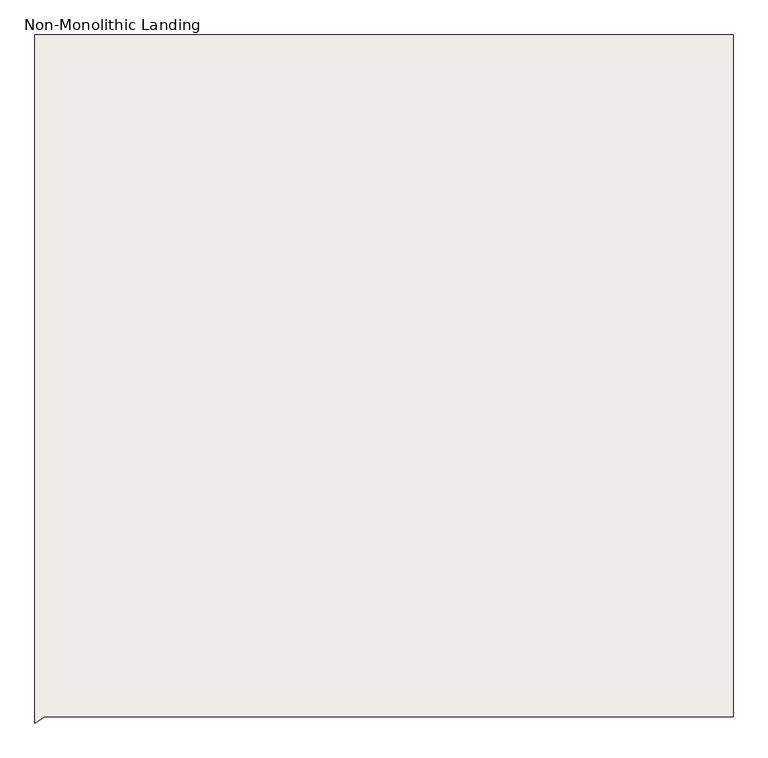
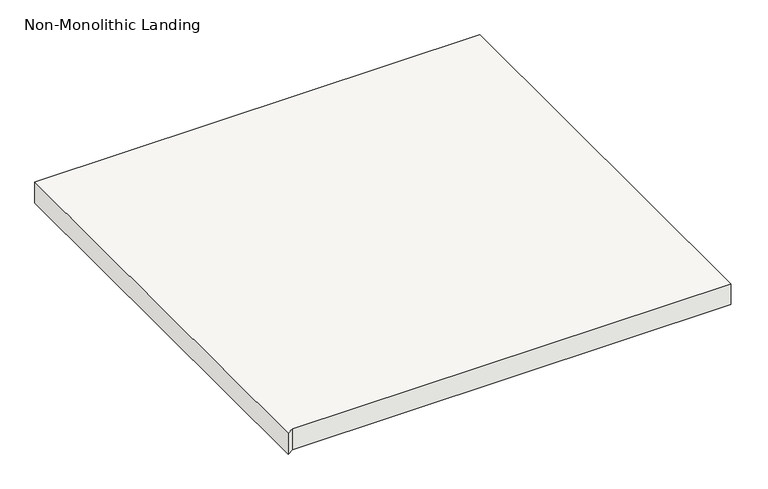
"""IFC4 building model written with IfcOpenShell, lengths in millimetres: slab geometry, Non-Monolithic Landing."""

from ifc_helpers import new_model, si_unit, frame, origin, place, context, project, spatial, polyline, outline, extrude, source, transform, mapped, element, save


def non_monolithic_landing_c08c66cc(model_context):
    return source(origin(), model_context, "Body", "SweptSolid", [
        extrude(outline(polyline([(-10492.1794909, -1507.9618509), (-9477.5794909, -1507.9618509), (-9477.5794909, -2498.5618509), (-10477.6052721, -2498.5618509), (-10492.1794909, -2507.9876321), (-10492.1794909, -1507.9618509)])), frame((0.0, 0.0, 4468.2117647), z_axis=(0.0, 0.0, 1.0), x_axis=(1.0, 0.0, 0.0)), (0.0, 0.0, 1.0), 50.0),
    ])


if __name__ == "__main__":
    model = new_model("IFC4")
    model_context = context("Model", 3, world=origin())
    ifc_project = project(units=[si_unit("LENGTHUNIT", "METRE", prefix="MILLI")], contexts=[model_context])
    site = spatial("IfcSite", under=ifc_project)
    building = spatial("IfcBuilding", under=site)
    placement = place(None, origin())
    non_monolithic_landing_shape = non_monolithic_landing_c08c66cc(model_context)
    element("IfcSlab", 1, ObjectType="Non-Monolithic Landing", at=placement, inside=building, context=model_context, shape_type="MappedRepresentation", body=[
        mapped(non_monolithic_landing_shape, transform((0.0, 0.0, 0.0), x_axis=(1.0, 0.0, 0.0), y_axis=(0.0, 1.0, 0.0), z_axis=(0.0, 0.0, 1.0))),
    ])
    save(model, "model.ifc")
